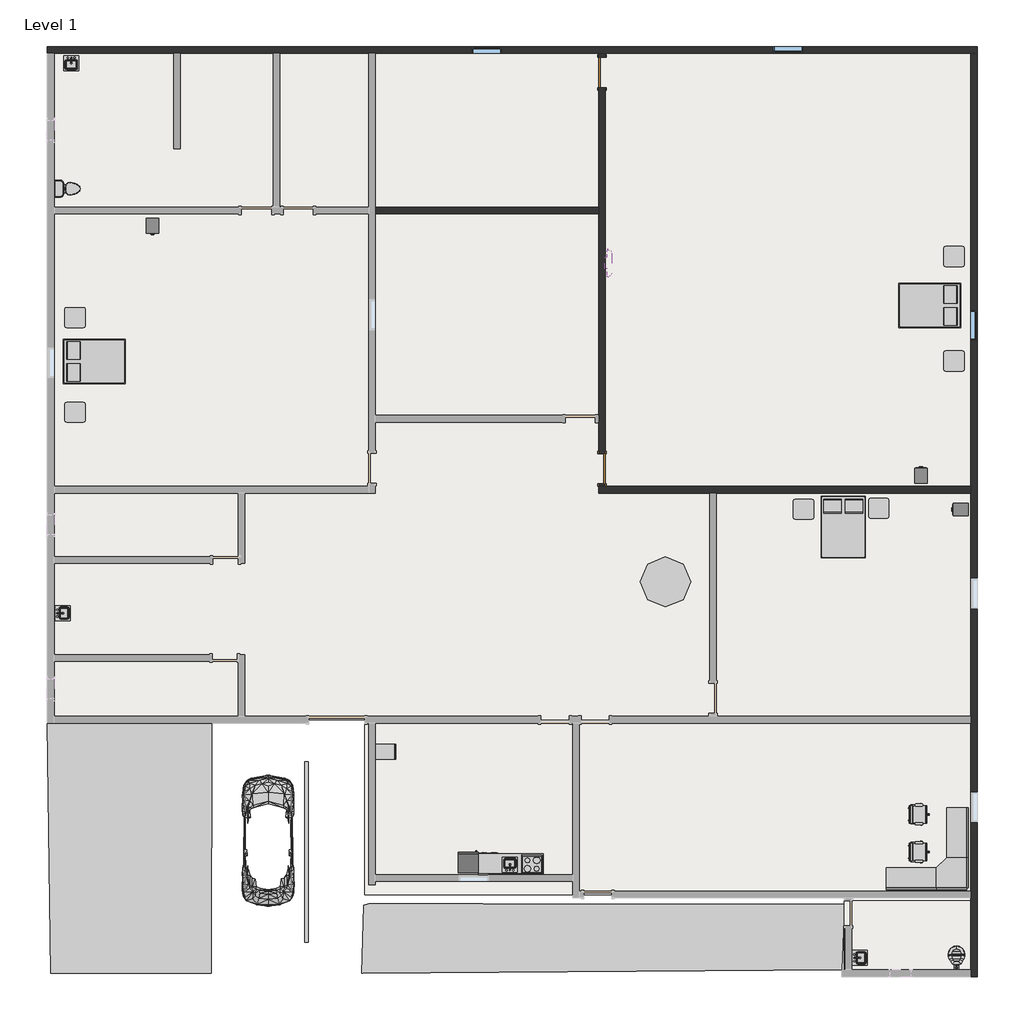
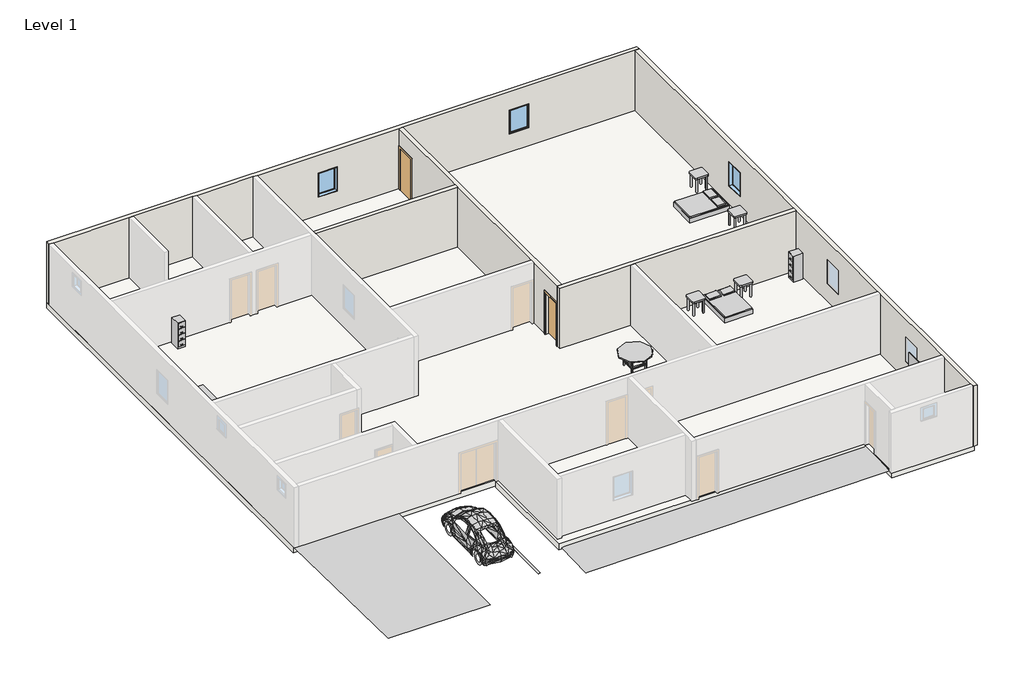
# One storey, part 2 of 2: 18 furniture elements, 9 proxies, 6 flow terminals, 5 walls, 3 slabs, 3 windows, 2 doors.
"""IFC4 building model written with IfcOpenShell, lengths in millimetres."""

from ifc_helpers import new_model, si_unit, frame, origin, origin_with_axes, place, context, project, spatial, polyline, outline, extrude, faceted_brep, triangles, transform, mapped, element, save
from components import proxy_7e1014cc, proxy_a6faaae8, proxy_45b28599, kitchenette_medium_kitchenette_medium_844211aa, parking_space_9_x_18_90_deg_b8b21359, rpc_beetle_rpc_beetle_3ce7ba48, proxy_c523a7b7, door_54dd4da4, flow_terminal_871c2e40, flow_terminal_bd37145e, toilet_domestic_3d_toilet_domestic_3d_f7549cf7, toilet_domestic_3d_toilet_domestic_3d_183bbd19, furniture_c8abb964, furniture_b1353b55, chair_task_arms_chair_task_arms_fa5a08ef, furniture_c6510c7c, furniture_56245f3a, furniture_bbcc68ce, furniture_bcf351fa, furniture_45e3acac, window_e2841890

model = new_model("IFC4")

# Units and contexts
model_context = context("Model", 3, world=origin())
ifc_project = project(units=[si_unit("LENGTHUNIT", "METRE", prefix="MILLI")], contexts=[model_context])

# Site, building, storey
site = spatial("IfcSite", under=ifc_project)
building = spatial("IfcBuilding", under=site)
storey = spatial("IfcBuildingStorey", under=building, Name="Level 1", Elevation=0.0)

# Proxies
placement = place(None, origin())
element("IfcBuildingElementProxy", 1, Name="Building Element Proxy", at=placement, inside=storey, context=model_context, shape_type="Tessellation", body=[
    triangles([(-16194.2719849, -5071.3753326, 0.0), (-16092.6723724, -12665.9757202, 0.0), (-11215.8723724, -12665.9757202, 0.0), (-11200.4547089, -5071.3753326, 0.0)], [[1, 2, 4], [3, 4, 2]], closed=False),
])
element("IfcBuildingElementProxy", 2, Name="Building Element Proxy", at=placement, inside=storey, context=model_context, shape_type="Tessellation", body=[
    triangles([(-6587.363031, -10707.5871185, 0.0), (-6648.5029037, -12665.9757202, 0.0), (7820.6964706, -10634.9136475, 0.0), (7935.72724, -12564.3749451, 0.0), (8011.92724, -10651.2591614, 0.0), (8011.92724, -10595.9078888, 0.0), (3816.6426178, -10588.5769409, 0.0), (369.9064911, -10591.2511963, 0.0), (-926.9083935, -10578.4368622, 0.0), (-2963.6249176, -10563.2447662, 0.0), (-6594.0672729, -10602.383075, 0.0), (-6377.0014526, -10588.111853, 0.0), (-6433.0230331, -10561.0297852, 0.0), (6685.585524, -10582.0401306, 0.0), (7909.8869568, -10585.3817871, 0.0), (8011.92724, -10564.8807129, 0.0)], [[11, 2, 1], [11, 1, 13], [2, 12, 1], [2, 4, 8], [8, 9, 2], [13, 12, 10], [12, 13, 1], [10, 9, 16], [10, 12, 2], [2, 9, 10], [13, 10, 16], [8, 7, 9], [3, 4, 5], [4, 3, 14], [3, 5, 15], [4, 7, 8], [15, 5, 6], [7, 14, 16], [7, 4, 14], [15, 16, 14], [16, 15, 6], [3, 15, 14], [7, 16, 9]], closed=False),
])
proxy_shape = proxy_7e1014cc(model_context)
element("IfcBuildingElementProxy", 3, Name="18\" x 24\" x 34 1/2\"", ObjectType="18\" x 24\" x 34 1/2\"", at=placement, inside=storey, context=model_context, shape_type="MappedRepresentation", body=[
    mapped(proxy_shape, transform((-5666.2229443, -6241.0928693, 0.0), x_axis=(0.0, 1.0000000000000002, 0.0), y_axis=(-1.0000000000000002, 0.0, 0.0), z_axis=(0.0, 0.0, 1.0))),
])
proxy_2_shape = proxy_a6faaae8(model_context)
element("IfcBuildingElementProxy", 4, Name="Cook Top-4 Unit2 : 22\" x 20\"", ObjectType="Cook Top-4 Unit2 : 22\" x 20\"", at=placement, inside=storey, context=model_context, shape_type="MappedRepresentation", body=[
    mapped(proxy_2_shape, transform((-1474.9725091, -9363.9754008, 0.0), x_axis=(-1.0000000000000004, 0.0, 0.0), y_axis=(0.0, -1.0000000000000004, 0.0), z_axis=(0.0, 0.0, 1.0))),
])
proxy_3_shape = proxy_45b28599(model_context)
element("IfcBuildingElementProxy", 5, Name="Dishwasher : 24\" x 24\" x 34\"", ObjectType="Dishwasher : 24\" x 24\" x 34\"", at=placement, inside=storey, context=model_context, shape_type="MappedRepresentation", body=[
    mapped(proxy_3_shape, transform((-2426.1550406, -9072.125836, 0.0), x_axis=(-1.0000000000000004, 0.0, 0.0), y_axis=(0.0, -1.0000000000000004, 0.0), z_axis=(0.0, 0.0, 1.0))),
])
kitchenette_medium_kitchenette_medium_shape = kitchenette_medium_kitchenette_medium_844211aa(model_context)
element("IfcBuildingElementProxy", 6, Name="Kitchenette - Medium : Kitchenette - Medium", ObjectType="Kitchenette - Medium : Kitchenette - Medium", at=placement, inside=storey, context=model_context, shape_type="MappedRepresentation", body=[
    mapped(kitchenette_medium_kitchenette_medium_shape, transform((-1799.1348042, -9668.7754008, 0.0), x_axis=(-1.0000000000000004, 0.0, 0.0), y_axis=(0.0, -1.0000000000000004, 0.0), z_axis=(0.0, 0.0, 1.0))),
])
parking_space_9_x_18_90_deg_shape = parking_space_9_x_18_90_deg_b8b21359(model_context)
element("IfcBuildingElementProxy", 7, Name="Parking Space : 9' x 18' - 90 deg", ObjectType="Parking Space : 9' x 18' - 90 deg", at=placement, inside=storey, context=model_context, shape_type="MappedRepresentation", body=[
    mapped(parking_space_9_x_18_90_deg_shape, transform((-8320.2725091, -11726.1754008, 0.0), x_axis=(-1.0000000000000004, 0.0, 0.0), y_axis=(0.0, -1.0000000000000004, 0.0), z_axis=(0.0, 0.0, 1.0))),
])
rpc_beetle_rpc_beetle_shape = rpc_beetle_rpc_beetle_3ce7ba48(model_context)
element("IfcBuildingElementProxy", 8, Name="RPC Beetle : RPC Beetle", ObjectType="RPC Beetle : RPC Beetle", at=placement, inside=storey, context=model_context, shape_type="MappedRepresentation", body=[
    mapped(rpc_beetle_rpc_beetle_shape, transform((-9488.6725091, -9871.9754008, 0.0), x_axis=(1.0, 0.0, 0.0), y_axis=(0.0, 1.0, 0.0), z_axis=(0.0, 0.0, 1.0))),
])
proxy_4_shape = proxy_c523a7b7(model_context)
element("IfcBuildingElementProxy", 9, Name="Refrigerator : 24\" x 25\" LH", ObjectType="Refrigerator : 24\" x 25\" LH", at=placement, inside=storey, context=model_context, shape_type="MappedRepresentation", body=[
    mapped(proxy_4_shape, transform((-3411.7225091, -9318.3264293, 0.0), x_axis=(-1.0000000000000004, 0.0, 0.0), y_axis=(0.0, -1.0000000000000004, 0.0), z_axis=(0.0, 0.0, 1.0))),
])

# Doors
door_shape = door_54dd4da4(model_context)
element("IfcDoor", 10, ObjectType="Single-Flush : 36\" x 84\"", at=placement, inside=storey, context=model_context, shape_type="MappedRepresentation", body=[
    mapped(door_shape, transform((645.9274909, 14689.8245992, 0.0), x_axis=(0.0, 1.0, 0.0), y_axis=(-1.0, 0.0, 0.0), z_axis=(0.0, 0.0, 1.0))),
])
element("IfcDoor", 11, ObjectType="Single-Flush : 36\" x 84\"", at=placement, inside=storey, context=model_context, shape_type="MappedRepresentation", body=[
    mapped(door_shape, transform((645.9274909, 2650.2245992, 0.0), x_axis=(0.0, -1.0, 0.0), y_axis=(1.0, 0.0, 0.0), z_axis=(0.0, 0.0, 1.0))),
])

# Flow terminals
flow_terminal_shape = flow_terminal_871c2e40(model_context)
element("IfcFlowTerminal", 12, ObjectType="Sink Kitchen-Island : 18\" x 18\"", at=placement, inside=storey, context=model_context, shape_type="MappedRepresentation", body=[
    mapped(flow_terminal_shape, transform((-15486.0617497, 14966.8791981, 0.0), x_axis=(1.0, 0.0, 0.0), y_axis=(0.0, 1.0, 0.0), z_axis=(0.0, 0.0, 1.0))),
])
element("IfcFlowTerminal", 13, ObjectType="Sink Kitchen-Island : 18\" x 18\"", at=placement, inside=storey, context=model_context, shape_type="MappedRepresentation", body=[
    mapped(flow_terminal_shape, transform((-15722.027108, -1746.9646413, 0.0), x_axis=(0.0, 1.0000000000000002, 0.0), y_axis=(-1.0000000000000002, 0.0, 0.0), z_axis=(0.0, 0.0, 1.0))),
])
element("IfcFlowTerminal", 14, ObjectType="Sink Kitchen-Island : 18\" x 18\"", at=placement, inside=storey, context=model_context, shape_type="MappedRepresentation", body=[
    mapped(flow_terminal_shape, transform((8484.172892, -12211.7646413, 0.0), x_axis=(0.0, 1.0000000000000002, 0.0), y_axis=(-1.0000000000000002, 0.0, 0.0), z_axis=(0.0, 0.0, 1.0))),
])
element("IfcFlowTerminal", 15, ObjectType="Sink Kitchen-Island : 18\" x 18\"", at=placement, inside=storey, context=model_context, shape_type="MappedRepresentation", body=[
    mapped(flow_terminal_shape, transform((-2132.3832686, -9361.6299997, -14.4), x_axis=(-1.0000000000000004, 0.0, 0.0), y_axis=(0.0, -1.0000000000000004, 0.0), z_axis=(0.0, 0.0, 1.0))),
])
flow_terminal_2_shape = flow_terminal_bd37145e(model_context)
element("IfcFlowTerminal", 16, ObjectType="Toilet-Commercial-Wall-3D : 15\" Seat Height", at=placement, inside=storey, context=model_context, shape_type="MappedRepresentation", body=[
    mapped(flow_terminal_2_shape, transform((11010.6243371, -12665.9754008, 0.0), x_axis=(1.0, 0.0, 0.0), y_axis=(0.0, 1.0, 0.0), z_axis=(0.0, 0.0, 1.0))),
])
toilet_domestic_3d_toilet_domestic_3d_shape = toilet_domestic_3d_toilet_domestic_3d_f7549cf7(model_context)
toilet_domestic_3d_toilet_domestic_3d_2_shape = toilet_domestic_3d_toilet_domestic_3d_183bbd19(model_context)
element("IfcFlowTerminal", 17, ObjectType="Toilet-Domestic-3D : Toilet-Domestic-3D", at=placement, inside=storey, context=model_context, shape_type="MappedRepresentation", body=[
    mapped(toilet_domestic_3d_toilet_domestic_3d_shape, transform((-15496.3764818, 11159.2245992, 0.0), x_axis=(0.0, 1.0000000000000002, 0.0), y_axis=(-1.0000000000000002, 0.0, 0.0), z_axis=(0.0, 0.0, 1.0))),
    mapped(toilet_domestic_3d_toilet_domestic_3d_2_shape, transform((-15496.3764818, 11159.2245992, 0.0), x_axis=(0.0, 1.0000000000000002, 0.0), y_axis=(-1.0000000000000002, 0.0, 0.0), z_axis=(0.0, 0.0, 1.0))),
])

# Furniture
furniture_shape = furniture_c8abb964(model_context)
element("IfcFurniture", 18, ObjectType="Bed-Box : Double 53\" x 74\"", at=placement, inside=storey, context=model_context, shape_type="MappedRepresentation", body=[
    mapped(furniture_shape, transform((-15006.3020173, 5574.9721402, 0.0), x_axis=(0.0, 1.0, 0.0), y_axis=(-1.0, 0.0, 0.0), z_axis=(0.0, 0.0, 1.0))),
])
element("IfcFurniture", 19, ObjectType="Bed-Box : Double 53\" x 74\"", at=placement, inside=storey, context=model_context, shape_type="MappedRepresentation", body=[
    mapped(furniture_shape, transform((10837.1569991, 7955.0770582, 0.0), x_axis=(0.0, -1.0000000000000002, 0.0), y_axis=(1.0000000000000002, 0.0, 0.0), z_axis=(0.0, 0.0, 1.0))),
])
element("IfcFurniture", 20, ObjectType="Bed-Box : Double 53\" x 74\"", at=placement, inside=storey, context=model_context, shape_type="MappedRepresentation", body=[
    mapped(furniture_shape, transform((7636.7569991, 1122.4770582, 0.0), x_axis=(1.0000000000000007, 0.0, 0.0), y_axis=(0.0, 1.0000000000000007, 0.0), z_axis=(0.0, 0.0, 1.0))),
])
furniture_2_shape = furniture_b1353b55(model_context)
element("IfcFurniture", 21, ObjectType="Cabinet-File 4 Drawer : 15\" x 18\"", at=placement, inside=storey, context=model_context, shape_type="MappedRepresentation", body=[
    mapped(furniture_2_shape, transform((-12878.6760621, 10183.7588994, 0.0), x_axis=(1.0, 0.0, 0.0), y_axis=(0.0, 1.0, 0.0), z_axis=(0.0, 0.0, 1.0))),
])
element("IfcFurniture", 22, ObjectType="Cabinet-File 4 Drawer : 15\" x 18\"", at=placement, inside=storey, context=model_context, shape_type="MappedRepresentation", body=[
    mapped(furniture_2_shape, transform((10208.1310438, 2304.8902991, 0.0), x_axis=(-1.0000000000000002, 0.0, 0.0), y_axis=(0.0, -1.0000000000000002, 0.0), z_axis=(0.0, 0.0, 1.0))),
])
element("IfcFurniture", 23, ObjectType="Cabinet-File 4 Drawer : 15\" x 18\"", at=placement, inside=storey, context=model_context, shape_type="MappedRepresentation", body=[
    mapped(furniture_2_shape, transform((11684.661791, 1290.4281522, 0.0), x_axis=(0.0, -1.0, 0.0), y_axis=(1.0, 0.0, 0.0), z_axis=(0.0, 0.0, 1.0))),
])
chair_task_arms_chair_task_arms_shape = chair_task_arms_chair_task_arms_fa5a08ef(model_context)
element("IfcFurniture", 24, ObjectType="Chair-Task Arms : Chair-Task Arms", at=placement, inside=storey, context=model_context, shape_type="MappedRepresentation", body=[
    mapped(chair_task_arms_chair_task_arms_shape, transform((10228.1815892, -7698.9845811, 0.0), x_axis=(0.0, -1.0, 0.0), y_axis=(1.0, 0.0, 0.0), z_axis=(0.0, 0.0, 1.0))),
])
element("IfcFurniture", 25, ObjectType="Chair-Task Arms : Chair-Task Arms", at=placement, inside=storey, context=model_context, shape_type="MappedRepresentation", body=[
    mapped(chair_task_arms_chair_task_arms_shape, transform((10228.1815892, -8841.9845811, 0.0), x_axis=(0.0, -1.0, 0.0), y_axis=(1.0, 0.0, 0.0), z_axis=(0.0, 0.0, 1.0))),
])
furniture_3_shape = furniture_c6510c7c(model_context)
element("IfcFurniture", 26, ObjectType="Counter Top w Sink Hole : 24\" Depth", at=placement, inside=storey, context=model_context, shape_type="MappedRepresentation", body=[
    mapped(furniture_3_shape, transform((-2332.5348042, -9668.7754008, -14.4), x_axis=(-1.0000000000000004, 0.0, 0.0), y_axis=(0.0, -1.0000000000000004, 0.0), z_axis=(0.0, 0.0, 1.0))),
])
furniture_4_shape = furniture_56245f3a(model_context)
element("IfcFurniture", 27, ObjectType="TV - Flat Screen : 32\"", at=placement, inside=storey, context=model_context, shape_type="MappedRepresentation", body=[
    mapped(furniture_4_shape, transform((885.0544567, 8894.6800851, 1524.0), x_axis=(0.0, -1.0000000000000004, 0.0), y_axis=(1.0000000000000004, 0.0, 0.0), z_axis=(0.0, 0.0, 1.0))),
])
furniture_5_shape = furniture_bbcc68ce(model_context)
element("IfcFurniture", 28, ObjectType="Table-Dining Round w Chairs : 60\" Diameter", at=placement, inside=storey, context=model_context, shape_type="MappedRepresentation", body=[
    mapped(furniture_5_shape, transform((2472.6455237, -593.8967122, 0.0), x_axis=(1.0, 0.0, 0.0), y_axis=(0.0, 1.0, 0.0), z_axis=(0.0, 0.0, 1.0))),
])
furniture_6_shape = furniture_bcf351fa(model_context)
element("IfcFurniture", 29, ObjectType="Table-End : 24\" x 24\"", at=placement, inside=storey, context=model_context, shape_type="MappedRepresentation", body=[
    mapped(furniture_6_shape, transform((-15664.6061394, 7095.2245992, 0.0), x_axis=(1.0, 0.0, 0.0), y_axis=(0.0, 1.0, 0.0), z_axis=(0.0, 0.0, 1.0))),
])
element("IfcFurniture", 30, ObjectType="Table-End : 24\" x 24\"", at=placement, inside=storey, context=model_context, shape_type="MappedRepresentation", body=[
    mapped(furniture_6_shape, transform((-15664.6061394, 4225.0245992, 0.0), x_axis=(1.0, 0.0, 0.0), y_axis=(0.0, 1.0, 0.0), z_axis=(0.0, 0.0, 1.0))),
])
element("IfcFurniture", 31, ObjectType="Table-End : 24\" x 24\"", at=placement, inside=storey, context=model_context, shape_type="MappedRepresentation", body=[
    mapped(furniture_6_shape, transform((11030.7938606, 5774.4245992, 0.0), x_axis=(1.0, 0.0, 0.0), y_axis=(0.0, 1.0, 0.0), z_axis=(0.0, 0.0, 1.0))),
])
element("IfcFurniture", 32, ObjectType="Table-End : 24\" x 24\"", at=placement, inside=storey, context=model_context, shape_type="MappedRepresentation", body=[
    mapped(furniture_6_shape, transform((11030.7938606, 8949.4245992, 0.0), x_axis=(1.0, 0.0, 0.0), y_axis=(0.0, 1.0, 0.0), z_axis=(0.0, 0.0, 1.0))),
])
element("IfcFurniture", 33, ObjectType="Table-End : 24\" x 24\"", at=placement, inside=storey, context=model_context, shape_type="MappedRepresentation", body=[
    mapped(furniture_6_shape, transform((8744.7938606, 1304.0245992, 0.0), x_axis=(1.0, 0.0, 0.0), y_axis=(0.0, 1.0, 0.0), z_axis=(0.0, 0.0, 1.0))),
])
element("IfcFurniture", 34, ObjectType="Table-End : 24\" x 24\"", at=placement, inside=storey, context=model_context, shape_type="MappedRepresentation", body=[
    mapped(furniture_6_shape, transform((6458.7938606, 1278.6245992, 0.0), x_axis=(1.0, 0.0, 0.0), y_axis=(0.0, 1.0, 0.0), z_axis=(0.0, 0.0, 1.0))),
])
furniture_7_shape = furniture_45e3acac(model_context)
element("IfcFurniture", 35, ObjectType="Work Station Cubicle : 96\" x 96\"", at=placement, inside=storey, context=model_context, shape_type="MappedRepresentation", body=[
    mapped(furniture_7_shape, transform((11639.3957386, -10620.9984084, 0.0), x_axis=(-1.0000000000000004, 0.0, 0.0), y_axis=(0.0, -1.0000000000000004, 0.0), z_axis=(0.0, 0.0, 1.0))),
])

# Slabs
element("IfcSlab", 36, ObjectType="Generic - 12\"", at=placement, inside=storey, context=model_context, shape_type="SweptSolid", body=[
    extrude(outline(polyline([(11948.9274909, 15477.2245992), (11948.9274909, -4969.7754008), (-16194.2725091, -4969.7754008), (-16194.2725091, 15477.2245992), (11948.9274909, 15477.2245992)])), frame((0.0, 0.0, -304.8), z_axis=(0.0, 0.0, 1.0), x_axis=(1.0, 0.0, 0.0)), (0.0, 0.0, 1.0), 304.8),
])
element("IfcSlab", 37, ObjectType="Generic - 12\"", at=placement, inside=storey, context=model_context, shape_type="SweptSolid", body=[
    extrude(outline(polyline([(11948.9274909, -5071.3754008), (11948.9274909, -10278.3754008), (-6555.8725091, -10278.3754008), (-6555.8725091, -5071.3754008), (11948.9274909, -5071.3754008)])), frame((0.0, 0.0, -304.8), z_axis=(0.0, 0.0, 1.0), x_axis=(1.0, 0.0, 0.0)), (0.0, 0.0, 1.0), 304.8),
])
element("IfcSlab", 38, ObjectType="Generic - 12\"", at=placement, inside=storey, context=model_context, shape_type="SweptSolid", body=[
    extrude(outline(polyline([(11948.9274909, -10456.1754008), (11948.9274909, -12665.9754008), (8011.9274909, -12665.9754008), (8011.9274909, -10456.1754008), (11948.9274909, -10456.1754008)])), frame((0.0, 0.0, -304.8), z_axis=(0.0, 0.0, 1.0), x_axis=(1.0, 0.0, 0.0)), (0.0, 0.0, 1.0), 304.8),
])

# Walls
element("IfcWall", 39, ObjectType="Generic - 8\"", at=placement, inside=storey, context=model_context, shape_type="Brep", body=[
    faceted_brep([(-16194.2725091, 15274.0245992, 0.0), (-15991.0725091, 15274.0245992, 0.0), (-12358.8725091, 15274.0245992, 0.0), (-12155.6725091, 15274.0245992, 0.0), (-9336.2725091, 15274.0245992, 0.0), (-9133.0725091, 15274.0245992, 0.0), (-6440.6725091, 15274.0245992, 0.0), (-6237.4725091, 15274.0245992, 0.0), (544.3274909, 15274.0245992, 0.0), (747.5274909, 15274.0245992, 0.0), (11847.3274909, 15274.0245992, 0.0), (12050.5274909, 15274.0245992, 0.0), (12050.5274909, 15274.0245992, 3048.0), (11847.3274909, 15274.0245992, 3048.0), (747.5274909, 15274.0245992, 3048.0), (544.3274909, 15274.0245992, 3048.0), (-6237.4725091, 15274.0245992, 3048.0), (-6440.6725091, 15274.0245992, 3048.0), (-9133.0725091, 15274.0245992, 3048.0), (-9336.2725091, 15274.0245992, 3048.0), (-12155.6725091, 15274.0245992, 3048.0), (-12358.8725091, 15274.0245992, 3048.0), (-15991.0725091, 15274.0245992, 3048.0), (-16194.2725091, 15274.0245992, 3048.0), (5840.2274909, 15274.0245992, 2133.6), (6754.6274909, 15274.0245992, 2133.6), (6754.6274909, 15274.0245992, 914.4), (5840.2274909, 15274.0245992, 914.4), (-2389.3725091, 15274.0245992, 2133.6), (-2389.3725091, 15274.0245992, 914.4), (-3303.7725091, 15274.0245992, 914.4), (-3303.7725091, 15274.0245992, 2133.6), (-16194.2725091, 15477.2245992, 0.0), (-16194.2725091, 15477.2245992, 3048.0), (12050.5274909, 15477.2245992, 3048.0), (12050.5274909, 15477.2245992, 0.0), (5840.2274909, 15477.2245992, 2133.6), (5840.2274909, 15477.2245992, 914.4), (6754.6274909, 15477.2245992, 914.4), (6754.6274909, 15477.2245992, 2133.6), (-2389.3725091, 15477.2245992, 2133.6), (-3303.7725091, 15477.2245992, 2133.6), (-3303.7725091, 15477.2245992, 914.4), (-2389.3725091, 15477.2245992, 914.4)], [[[0, 1, 2, 3, 4, 5, 6, 7, 8, 9, 10, 11, 12, 13, 14, 15, 16, 17, 18, 19, 20, 21, 22, 23], [24, 25, 26, 27], [28, 29, 30, 31]], [[32, 33, 34, 35], [36, 37, 38, 39], [40, 41, 42, 43]], [[11, 10, 9, 8, 7, 6, 5, 4, 3, 2, 1, 0, 32, 35]], [[23, 22, 21, 20, 19, 18, 17, 16, 15, 14, 13, 12, 34, 33]], [[12, 11, 35, 34]], [[0, 23, 33, 32]], [[37, 36, 24, 27]], [[38, 37, 27, 26]], [[39, 38, 26, 25]], [[36, 39, 25, 24]], [[29, 28, 40, 43]], [[30, 29, 43, 42]], [[31, 30, 42, 41]], [[28, 31, 41, 40]]]),
])
element("IfcWall", 40, ObjectType="Generic - 8\"", at=placement, inside=storey, context=model_context, shape_type="Brep", body=[
    faceted_brep([(11847.3274909, 15274.0245992, 0.0), (11847.3274909, 2116.8245992, 0.0), (11847.3274909, 1913.6245992, 0.0), (11847.3274909, -4868.1754008, 0.0), (11847.3274909, -5071.3754008, 0.0), (11847.3274909, -10176.7754008, 0.0), (11847.3274909, -10379.9754008, 0.0), (11847.3274909, -12564.3754008, 0.0), (11847.3274909, -12767.5754008, 0.0), (11847.3274909, -12767.5754008, 3048.0), (11847.3274909, -12564.3754008, 3048.0), (11847.3274909, -10379.9754008, 3048.0), (11847.3274909, -10176.7754008, 3048.0), (11847.3274909, -5071.3754008, 3048.0), (11847.3274909, -4868.1754008, 3048.0), (11847.3274909, 1913.6245992, 3048.0), (11847.3274909, 2116.8245992, 3048.0), (11847.3274909, 15274.0245992, 3048.0), (11847.3274909, -7166.8754008, 2133.6), (11847.3274909, -8081.2754008, 2133.6), (11847.3274909, -8081.2754008, 914.4), (11847.3274909, -7166.8754008, 914.4), (11847.3274909, -677.1754008, 2133.6), (11847.3274909, -1591.5754008, 2133.6), (11847.3274909, -1591.5754008, 914.4), (11847.3274909, -677.1754008, 914.4), (11847.3274909, 6561.8245992, 2133.6), (11847.3274909, 6561.8245992, 914.4), (11847.3274909, 7476.2245992, 914.4), (11847.3274909, 7476.2245992, 2133.6), (12050.5274909, 15274.0245992, 0.0), (12050.5274909, 15274.0245992, 3048.0), (12050.5274909, -12767.5754008, 3048.0), (12050.5274909, -12767.5754008, 0.0), (12050.5274909, -7166.8754008, 2133.6), (12050.5274909, -7166.8754008, 914.4), (12050.5274909, -8081.2754008, 914.4), (12050.5274909, -8081.2754008, 2133.6), (12050.5274909, -677.1754008, 2133.6), (12050.5274909, -677.1754008, 914.4), (12050.5274909, -1591.5754008, 914.4), (12050.5274909, -1591.5754008, 2133.6), (12050.5274909, 6561.8245992, 2133.6), (12050.5274909, 7476.2245992, 2133.6), (12050.5274909, 7476.2245992, 914.4), (12050.5274909, 6561.8245992, 914.4)], [[[0, 1, 2, 3, 4, 5, 6, 7, 8, 9, 10, 11, 12, 13, 14, 15, 16, 17], [18, 19, 20, 21], [22, 23, 24, 25], [26, 27, 28, 29]], [[30, 31, 32, 33], [34, 35, 36, 37], [38, 39, 40, 41], [42, 43, 44, 45]], [[8, 7, 6, 5, 4, 3, 2, 1, 0, 30, 33]], [[17, 16, 15, 14, 13, 12, 11, 10, 9, 32, 31]], [[0, 17, 31, 30]], [[9, 8, 33, 32]], [[35, 34, 18, 21]], [[36, 35, 21, 20]], [[37, 36, 20, 19]], [[34, 37, 19, 18]], [[39, 38, 22, 25]], [[40, 39, 25, 24]], [[41, 40, 24, 23]], [[38, 41, 23, 22]], [[27, 26, 42, 45]], [[28, 27, 45, 44]], [[29, 28, 44, 43]], [[26, 29, 43, 42]]]),
])
element("IfcWall", 41, ObjectType="Generic - 8\"", at=placement, inside=storey, context=model_context, shape_type="Brep", body=[
    faceted_brep([(544.3274909, 1913.6245992, 0.0), (3922.5274909, 1913.6245992, 0.0), (4125.7274909, 1913.6245992, 0.0), (11847.3274909, 1913.6245992, 0.0), (11847.3274909, 1913.6245992, 3048.0), (4125.7274909, 1913.6245992, 3048.0), (3922.5274909, 1913.6245992, 3048.0), (544.3274909, 1913.6245992, 3048.0), (544.3274909, 2116.8245992, 0.0), (544.3274909, 2116.8245992, 3048.0), (747.5274909, 2116.8245992, 3048.0), (11847.3274909, 2116.8245992, 3048.0), (11847.3274909, 2116.8245992, 0.0), (747.5274909, 2116.8245992, 0.0)], [[[0, 1, 2, 3, 4, 5, 6, 7]], [[8, 9, 10, 11, 12, 13]], [[3, 2, 1, 0, 8, 13, 12]], [[7, 6, 5, 4, 11, 10, 9]], [[4, 3, 12, 11]], [[0, 7, 9, 8]]]),
])
element("IfcWall", 42, ObjectType="Generic - 8\"", at=placement, inside=storey, context=model_context, shape_type="Brep", body=[
    faceted_brep([(544.3274909, 2193.0245992, 2133.6), (544.3274909, 2193.0245992, 0.0), (544.3274909, 2116.8245992, 0.0), (544.3274909, 2116.8245992, 3048.0), (544.3274909, 4072.6245992, 3048.0), (544.3274909, 4275.8245992, 3048.0), (544.3274909, 10397.2245992, 3048.0), (544.3274909, 10600.4245992, 3048.0), (544.3274909, 15274.0245992, 3048.0), (544.3274909, 15274.0245992, 0.0), (544.3274909, 15147.0245992, 0.0), (544.3274909, 15147.0245992, 2133.6), (544.3274909, 14232.6245992, 2133.6), (544.3274909, 14232.6245992, 0.0), (544.3274909, 10600.4245992, 0.0), (544.3274909, 10397.2245992, 0.0), (544.3274909, 4275.8245992, 0.0), (544.3274909, 4072.6245992, 0.0), (544.3274909, 3107.4245992, 0.0), (544.3274909, 3107.4245992, 2133.6), (747.5274909, 2116.8245992, 0.0), (747.5274909, 2193.0245992, 0.0), (747.5274909, 2193.0245992, 2133.6), (747.5274909, 3107.4245992, 2133.6), (747.5274909, 3107.4245992, 0.0), (747.5274909, 14232.6245992, 0.0), (747.5274909, 14232.6245992, 2133.6), (747.5274909, 15147.0245992, 2133.6), (747.5274909, 15147.0245992, 0.0), (747.5274909, 15274.0245992, 0.0), (747.5274909, 15274.0245992, 3048.0), (747.5274909, 2116.8245992, 3048.0)], [[[0, 1, 2, 3, 4, 5, 6, 7, 8, 9, 10, 11, 12, 13, 14, 15, 16, 17, 18, 19]], [[20, 21, 22, 23, 24, 25, 26, 27, 28, 29, 30, 31]], [[29, 28, 10, 9]], [[2, 1, 21, 20]], [[18, 17, 16, 15, 14, 13, 25, 24]], [[8, 7, 6, 5, 4, 3, 31, 30]], [[3, 2, 20, 31]], [[9, 8, 30, 29]], [[11, 10, 28, 27]], [[12, 11, 27, 26]], [[13, 12, 26, 25]], [[22, 21, 1, 0]], [[23, 22, 0, 19]], [[24, 23, 19, 18]]]),
])
element("IfcWall", 43, ObjectType="Generic - 8\"", at=placement, inside=storey, context=model_context, shape_type="SweptSolid", body=[
    extrude(outline(polyline([(544.3274909, 10397.2245992), (-6237.4725091, 10397.2245992), (-6237.4725091, 10600.4245992), (544.3274909, 10600.4245992), (544.3274909, 10397.2245992)])), origin_with_axes(), (0.0, 0.0, 1.0), 3048.0),
])

# Windows
window_shape = window_e2841890(model_context)
element("IfcWindow", 44, ObjectType="Fixed : 36\" x 48\"", at=placement, inside=storey, context=model_context, shape_type="MappedRepresentation", body=[
    mapped(window_shape, transform((11948.9274909, 6980.9245992, 0.0), x_axis=(0.0, -1.0, 0.0), y_axis=(1.0, 0.0, 0.0), z_axis=(0.0, 0.0, 1.0))),
])
element("IfcWindow", 45, ObjectType="Fixed : 36\" x 48\"", at=placement, inside=storey, context=model_context, shape_type="MappedRepresentation", body=[
    mapped(window_shape, transform((6259.3274909, 15375.6245992, 0.0), x_axis=(-1.0, 0.0, 0.0), y_axis=(0.0, -1.0, 0.0), z_axis=(0.0, 0.0, 1.0))),
])
element("IfcWindow", 46, ObjectType="Fixed : 36\" x 48\"", at=placement, inside=storey, context=model_context, shape_type="MappedRepresentation", body=[
    mapped(window_shape, transform((-2808.4725091, 15375.6245992, 0.0), x_axis=(1.0, 0.0, 0.0), y_axis=(0.0, 1.0, 0.0), z_axis=(0.0, 0.0, 1.0))),
])

save(model, "model.ifc")

# Revit data of these elements
# Type "18\" x 24\" x 34 1/2\""
#   Label = "T"
#   Assembly Code = "E1090400"
#   Depth = 2' - 0"
#   Height = 2' - 10 1/2"
#   Width = 1' - 6"
#   Panel Face Material = Plastic, Opaque Black
#   Trach Compact. Material = Steel, Paint Finish, Ivory, Matte
#   Default Elevation = 0
# Type "Cook Top-4 Unit2 : 22\" x 20\""
#   Depth = 1' - 8"
#   Width = 1' - 10"
#   Burner Material = Steel, Chrome Plated
#   Cooktop Material = Steel, Polished
#   Default Elevation = 0
#   Assembly Code = ""
# Type "Dishwasher : 24\" x 24\" x 34\""
#   Label = "DW"
#   Assembly Code = "E1090400"
#   Depth = 2' - 0"
#   Height = 2' - 10"
#   Width = 2' - 0"
#   Dishwasher Material = Steel, Paint Finish, Ivory, Glossy
#   Panel Face Material = Plastic, Opaque Black
#   Default Elevation = 0
# Type "Kitchenette - Medium : Kitchenette - Medium"
#   Assembly Code = "E1090400"
#   Counter Length = 6' - 6"
#   Cabinet Width = 4' - 6"
#   Cabinet Height = 2' - 10 1/2"
#   Cabinet Depth = 2' - 0"
#   Toe Depth = 0' - 3"
#   Toe Height = 0' - 3 1/2"
#   Cabinet Material = Cabinets
#   Door/Drawer Material = Cabinets
#   Handle Material = Cabinets - Handles
#   Default Elevation = 0
# Type "Parking Space : 9' x 18' - 90 deg"
#   Angle = 90.00°
#   Parking Length = 18' - 0"
#   Parking Width = 9' - 0"
#   pl = 18' - 0"
#   pw = 9' - 0"
# Type "RPC Beetle : RPC Beetle"
#   built-in parameter 1005195 = "RPC-16-0U6E-L4EG-ENH1-J3KF-SVEL-0TX4-C0"
#   Height = 0
# Type "Refrigerator : 24\" x 25\" LH"
#   Label = "REF."
#   Assembly Code = "E1090400"
#   Depth = 2' - 0 3/4"
#   Handle = 0' - 1 1/2"
#   Height = 5' - 3 1/2"
#   Rear Clearance = 0' - 2"
#   Top Door Height = 1' - 8"
#   Width = 1' - 11 1/2"
#   Material = Steel, Paint Finish, Ivory, Glossy
#   Default Elevation = 0
# Type "Single-Flush : 36\" x 84\""
#   Type Mark = "1"
#   Construction Type Id = "MDOOR"
#   Assembly Code = "C1020"
#   Analytic Construction = "Metal"
#   Thickness = 0' - 2"
#   Heat Transfer Coefficient (U) = 0.651978 BTU/(h·ft²·°F)
#   Height = 7' - 0"
#   Trim Projection Ext = 0' - 1"
#   Trim Projection Int = 0' - 1"
#   Trim Width = 0' - 3"
#   Width = 3' - 0"
#   Define Thermal Properties by = 1
#   Door Material = Door - Panel
#   Frame Material = Door - Frame
#   Visual Light Transmittance = 0
#   Solar Heat Gain Coefficient = 0
#   Function = (empty or 0)
#   Wall Closure = (empty or 0)
# Type "Sink Kitchen-Island : 18\" x 18\""
#   Assembly Code = "D2010410"
#   Counter Height = 3' - 0"
#   Depth = 1' - 6"
#   Width = 1' - 6"
#   Faucet Material = Steel, Polished
#   Sink Material = Steel, Polished
#   Default Elevation = 0
# Type "Toilet-Commercial-Wall-3D : 15\" Seat Height"
#   Assembly Code = "D2010110"
#   Mounting Height = 1' - 3"
#   Piping Material = Steel, Polished
#   Toilet - Bowl Material = Porcelain, Ivory
#   Toilet - Seat Material = Laminate, Ivory, Matte
#   Default Elevation = 0
# Type "Toilet-Domestic-3D : Toilet-Domestic-3D"
#   Assembly Code = "D2010110"
#   Toilet - Bowl/Basin Material = Porcelain, Linen
#   Toilet - Seat Material = Laminate, Linen, Matte
#   Default Elevation = 0
# Type "Bed-Box : Double 53\" x 74\""
#   Assembly Code = "E2020200"
#   Length = 6' - 2"
#   Width = 4' - 5"
#   Frame Material = Birch
#   Mattress Material = Linen, White
#   Default Elevation = 0
# Type "Cabinet-File 4 Drawer : 15\" x 18\""
#   Assembly Code = "E2020200"
#   Depth = 1' - 6"
#   Height = 4' - 4"
#   Width = 1' - 3"
#   Cabinet Material = Steel, Paint Finish, Ivory, Glossy
#   Handle Material = Steel, Chrome Plated
#   Default Elevation = 0
# Type "Chair-Task Arms : Chair-Task Arms"
#   Assembly Code = "E2020200"
#   Base Material = Plastic, Opaque Black
#   Caster Material = Plastic, Opaque Black
#   Seat/Back Material = Textile - Slate Blue
#   Default Elevation = 0
# Type "Counter Top w Sink Hole : 24\" Depth"
#   Assembly Code = "C1030400"
#   Counter Thickness = 0' - 1 1/2"
#   Depth = 2' - 1"
#   Height = 3' - 0"
#   Length [instance default] = 8' - 0"
#   Sink Location [instance default] = 2' - 0"
#   Sink Location To Wall [instance default] = 0' - 6"
#   Sink Opening Depth [instance default] = 1' - 3"
#   Sink Opening Width [instance default] = 2' - 3"
#   Counter Top Material = none
#   Default Elevation = 0
# Type "TV - Flat Screen : 32\""
#   SinAng = 0' - 0.0193"
#   L = 2' - 3.79372"
#   H = 1' - 3.6354"
#   Thickness = 0' - 4.33071"
#   Diagonal = 2' - 7.88976"
#   CosAng = 0' - 0.03431"
#   Stand [instance default] = yes
#   Default Elevation = 0
# Type "Table-Dining Round w Chairs : 60\" Diameter"
#   Assembly Code = "E2020200"
#   Radius = 2' - 6"
#   Diameter = 5' - 0"
#   Height = 2' - 6"
#   Chairs = 6
#   Base Material = Pine
#   Top Material = Laminate, Linen, Matte
#   Default Elevation = 0
# Type "Table-End : 24\" x 24\""
#   Assembly Code = "E2020200"
#   Height = 2' - 6"
#   Length = 2' - 0"
#   Width = 2' - 0"
#   Base Material = Birch
#   Top Material = Laminate, Ivory, Matte
#   Default Elevation = 0
# Type "Work Station Cubicle : 96\" x 96\""
#   Assembly Code = "E2020"
#   Desktop Height = 2' - 6"
#   Desktop1 Width = 2' - 0"
#   Desktop2 Width = 2' - 0"
#   Panel Height = 5' - 6"
#   Panel1 Length = 5' - 0"
#   Panel2 Length = 5' - 0"
#   Cube Panel Material = Textile - Light Gray
#   Work Top Material = Laminate, Ivory, Matte
#   Default Elevation = 0
# Type "Generic - 12\""
#   Assembly Code = "B1010"
#   Function = 0
#   Layers, outside or top first: 1' - 0" no material (function 1)
# Type "Generic - 8\""
#   Assembly Code = "B2010"
#   Layers, outside or top first: 0' - 8" no material (function 1)
# Type "Fixed : 36\" x 48\""
#   Type Mark = "1"
#   Construction Type Id = "GSP4R"
#   Assembly Code = "B2020100"
#   Analytic Construction = "1/8 in Pilkington single glazing"
#   Visual Light Transmittance = 0.9
#   Solar Heat Gain Coefficient = 0.78
#   Heat Transfer Coefficient (U) = 0.6496 BTU/(h·ft²·°F)
#   Height = 4' - 0"
#   Default Sill Height = 3' - 0"
#   Width = 3' - 0"
#   Window Inset = 0' - 0 3/4"
#   Define Thermal Properties by = 1
#   Glass Pane Material = Glass
#   Sash Material = Sash
#   Wall Closure = (empty or 0)
# Elements 1, 2 (IfcBuildingElementProxy)
#   Material = none
#   Phase Created = New Construction
# Element 3 (IfcBuildingElementProxy, "18\" x 24\" x 34 1/2\"")
#   Phase Created = New Construction
#   Materials on its faces: "Steel, Paint Finish, Ivory, Matte", "Plastic, Opaque Black"
# Element 4 (IfcBuildingElementProxy, "Cook Top-4 Unit2 : 22\" x 20\"")
#   Phase Created = New Construction
#   Materials on its faces: "Steel, Chrome Plated", "Steel, Polished"
# Element 5 (IfcBuildingElementProxy, "Dishwasher : 24\" x 24\" x 34\"")
#   Phase Created = New Construction
#   Materials on its faces: "Steel, Paint Finish, Ivory, Glossy", "Plastic, Opaque Black"
# Element 6 (IfcBuildingElementProxy, "Kitchenette - Medium : Kitchenette - Medium")
#   Phase Created = New Construction
#   Materials on its faces: "Cabinets", "Cabinets - Handles"
# Element 7 (IfcBuildingElementProxy, "Parking Space : 9' x 18' - 90 deg")
#   Phase Created = New Construction
#   Materials on its faces: "Parking Stripe"
# Element 8 (IfcBuildingElementProxy, "RPC Beetle : RPC Beetle")
#   Phase Created = New Construction
# Element 9 (IfcBuildingElementProxy, "Refrigerator : 24\" x 25\" LH")
#   Phase Created = New Construction
#   Materials on its faces: "Steel, Paint Finish, Ivory, Glossy", "Steel, Chrome Plated"
# Elements 10, 11 (IfcDoor, "Single-Flush : 36\" x 84\"")
#   Phase Created = New Construction
#   Materials on its faces: "Door - Frame", "Door - Panel"
# Element 12 (IfcFlowTerminal, "Sink Kitchen-Island : 18\" x 18\"")
#   Mark = "2"
#   Phase Created = New Construction
#   Materials on its faces: "Steel, Polished"
# Element 13 (IfcFlowTerminal, "Sink Kitchen-Island : 18\" x 18\"")
#   Mark = "3"
#   Phase Created = New Construction
#   Materials on its faces: "Steel, Polished"
# Element 14 (IfcFlowTerminal, "Sink Kitchen-Island : 18\" x 18\"")
#   Mark = "4"
#   Phase Created = New Construction
#   Materials on its faces: "Steel, Polished"
# Element 15 (IfcFlowTerminal, "Sink Kitchen-Island : 18\" x 18\"")
#   Mark = "7"
#   Phase Created = New Construction
#   Materials on its faces: "Steel, Polished"
# Element 16 (IfcFlowTerminal, "Toilet-Commercial-Wall-3D : 15\" Seat Height")
#   Mark = "6"
#   Phase Created = New Construction
#   Materials on its faces: "Laminate, Ivory, Matte", "Porcelain, Ivory", "Steel, Polished"
# Element 17 (IfcFlowTerminal, "Toilet-Domestic-3D : Toilet-Domestic-3D")
#   Mark = "5"
#   Phase Created = New Construction
#   Materials on its faces: "Porcelain, Linen", "Laminate, Linen, Matte"
# Elements 18, 19, 20 (IfcFurniture, "Bed-Box : Double 53\" x 74\"")
#   Phase Created = New Construction
#   Materials on its faces: "Birch", "Linen, White"
# Elements 21, 22, 23 (IfcFurniture, "Cabinet-File 4 Drawer : 15\" x 18\"")
#   Phase Created = New Construction
#   Materials on its faces: "Steel, Chrome Plated", "Steel, Paint Finish, Ivory, Glossy"
# Elements 24, 25 (IfcFurniture, "Chair-Task Arms : Chair-Task Arms")
#   Phase Created = New Construction
#   Materials on its faces: "Plastic, Opaque Black", "Textile - Slate Blue"
# Element 26 (IfcFurniture, "Counter Top w Sink Hole : 24\" Depth")
#   Sink Opening Depth = 1' - 2"
#   Sink Location To Wall = 0' - 6"
#   Length = 6' - 6"
#   Sink Location = 3' - 4"
#   Sink Opening Width = 1' - 4"
#   Phase Created = New Construction
#   Materials on its faces: "Counter Top"
# Element 27 (IfcFurniture, "TV - Flat Screen : 32\"")
#   Stand = yes
#   Phase Created = New Construction
#   Materials on its faces: "TV - Black", "TV - Glass", "TV - Screen"
# Element 28 (IfcFurniture, "Table-Dining Round w Chairs : 60\" Diameter")
#   Phase Created = New Construction
#   Materials on its faces: "Pine", "Laminate, Linen, Matte"
# Elements 29, 30, 31, 32, 33, 34 (IfcFurniture, "Table-End : 24\" x 24\"")
#   Phase Created = New Construction
#   Materials on its faces: "Laminate, Ivory, Matte", "Birch"
# Element 35 (IfcFurniture, "Work Station Cubicle : 96\" x 96\"")
#   Phase Created = New Construction
#   Materials on its faces: "Textile - Light Gray", "Laminate, Ivory, Matte"
# Elements 36, 37, 38 (IfcSlab, "Generic - 12\"")
#   Height Offset From Level = 0' - 0"
#   Phase Created = New Construction
#   Materials on its faces: "Default Floor"
# Elements 39, 40, 41, 42, 43 (IfcWall, "Generic - 8\"")
#   Top Offset = 0' - 0"
#   Base Offset = 0' - 0"
#   Unconnected Height = 10' - 0"
#   wall height = 10' - 0"
#   Phase Created = New Construction
#   Base Constraint = Level 1
#   Materials on its faces: "Default Wall"
# Element 44 (IfcWindow, "Fixed : 36\" x 48\"")
#   Mark = "5"
#   Phase Created = New Construction
#   Materials on its faces: "Sash", "Glass"
# Element 45 (IfcWindow, "Fixed : 36\" x 48\"")
#   Mark = "6"
#   Phase Created = New Construction
#   Materials on its faces: "Sash", "Glass"
# Element 46 (IfcWindow, "Fixed : 36\" x 48\"")
#   Mark = "7"
#   Phase Created = New Construction
#   Materials on its faces: "Sash", "Glass"
# Materials
#   "Plastic, Opaque Black": class "Plastic", colour RGB 0 0 0, transparency 0.7, Description = "Plastic, generic, opaque black", Cost = 0
#   "Steel, Paint Finish, Ivory, Matte": class "Metal", colour RGB 247 247 239, transparency 0, Description = "Steel, paint finish, ivory, matte", Cost = 0
#   "Steel, Chrome Plated": class "Metal", colour RGB 17 17 17, transparency 0, Description = "Chromiuim plated steel", Cost = 0
#   "Steel, Polished": class "Metal", colour RGB 57 57 57, transparency 0, Description = "Polished steel", Cost = 0
#   "Steel, Paint Finish, Ivory, Glossy": class "Metal", colour RGB 247 247 239, transparency 0, Description = "Steel, paint finish, ivory, glossy", Cost = 0
#   "Cabinets": colour RGB 249 249 249, transparency 0
#   "Cabinets - Handles": class "Metal", colour RGB 57 57 57, transparency 0
#   "Door - Panel": class "Wood", colour RGB 210 159 95, transparency 0
#   "Door - Frame": colour RGB 118 70 51, transparency 0
#   "Porcelain, Ivory": class "Ceramic", colour RGB 247 247 239, transparency 0, Description = "Porcelain, ivory", Cost = 0
#   "Laminate, Ivory, Matte": class "Plastic", colour RGB 247 247 239, transparency 0, Description = "Plastic Laminate - Ivory, Matte", Cost = 0
#   "Porcelain, Linen": class "Ceramic", colour RGB 249 239 230, transparency 0, Description = "Porcelain, linen", Cost = 0
#   "Laminate, Linen, Matte": class "Plastic", colour RGB 249 239 230, transparency 0, Description = "Plastic Laminate - Linen, Matte", Cost = 0
#   "Birch": class "Wood", colour RGB 224 178 126, transparency 0, Description = "Betula Alleghaniensis", Cost = 0
#   "Linen, White": class "Textile", colour RGB 247 247 239, transparency 0, Description = "Linen, white", Cost = 0
#   "Textile - Slate Blue": class "Fabric", colour RGB 98 102 118, transparency 0
#   "Pine": class "Wood", colour RGB 223 192 134, transparency 0, Description = "Pinus Echinata", Cost = 0
#   "Textile - Light Gray": class "Fabric", colour RGB 204 204 204, transparency 0
#   "Glass": class "Glass", colour RGB 0 128 192, transparency 0.75, Description = "Soda Lime Glass", Cost = 0
#   "Sash": class "Wood", colour RGB 224 178 126, transparency 0
#   "Parking Stripe": class "Paint", colour RGB 250 250 91, transparency 0
#   "Counter Top": class "Wood", colour RGB 226 177 128, transparency 0
#   "TV - Black": colour RGB 49 49 49, transparency 0
#   "TV - Glass": colour RGB 157 157 157, transparency 0.9
#   "TV - Screen": colour RGB 0 0 0, transparency 0
#   "Default Floor": colour RGB 128 128 128, transparency 0
#   "Default Wall": colour RGB 128 128 128, transparency 0
